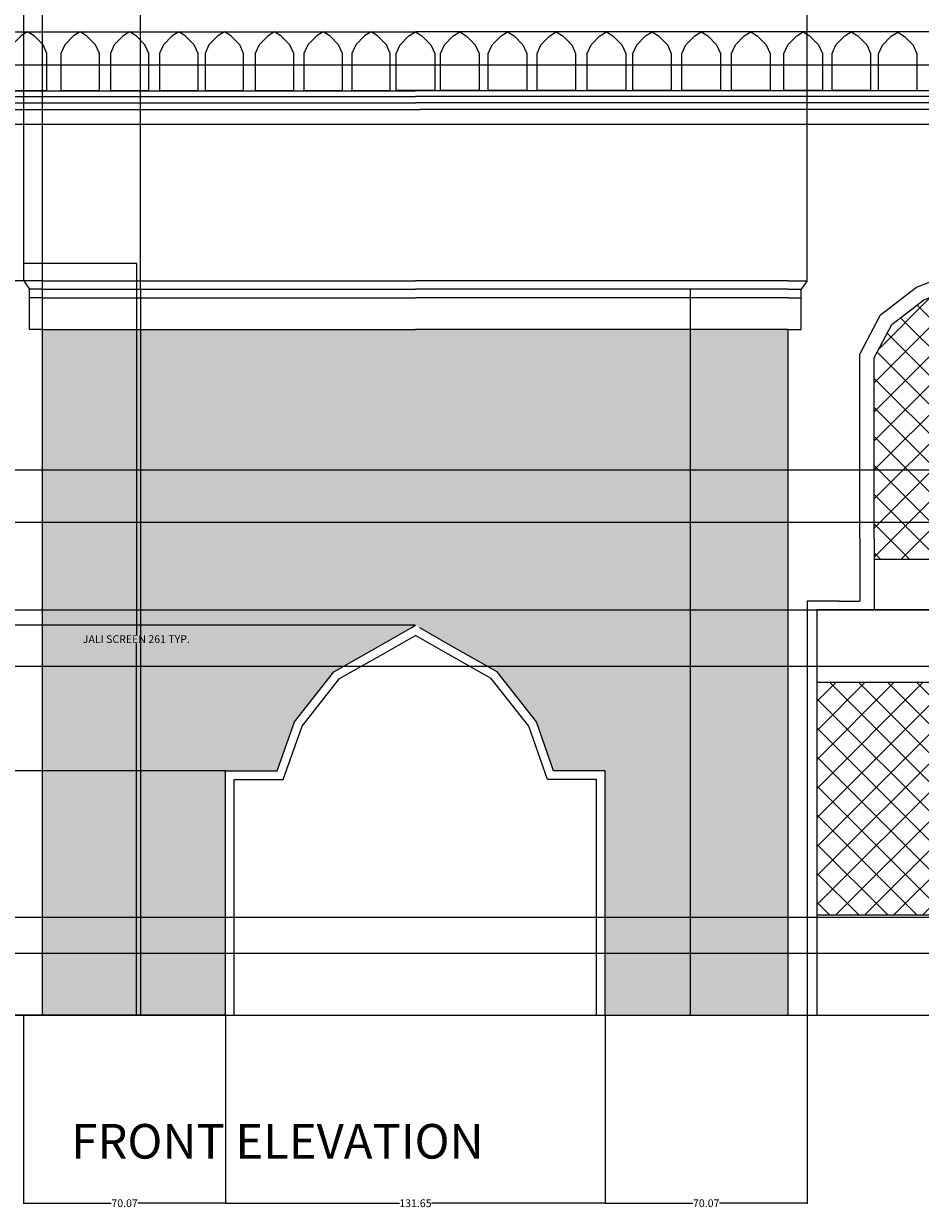
# Model space of a CAD drawing. Units: inches. Extents: x 2 to 1442, y 20 to 729.
# Tile 4 of 8: x 586 to 897, y 20 to 431. Entities that reach past the tile are written whole.
import ezdxf

# ---------------------------------------------------------------- set-up
doc = ezdxf.new("R2010")
doc.units = ezdxf.units.IN
doc.header["$MEASUREMENT"] = 0
for name, color, linetype, lineweight in [('A-ANNO-DIMS', 2, 'Continuous', 18), ('A-ANNO-TEXT', 7, 'Continuous', 25), ('A-ELEV', 7, 'Continuous', 25), ('A-GLAZ', 4, 'Continuous', 18), ('A-GLAZ-PATT', 9, 'Continuous', 13), ('A-WALL-PATT', 8, 'Continuous', 13)]:
    doc.layers.add(name, color=color, linetype=linetype, lineweight=lineweight)
doc.styles.get("Standard").update_dxf_attribs({"font": 'arial.ttf'})
doc.dimstyles.get("Standard").update_dxf_attribs({"dimtxt": 2.6875, "dimasz": 0.18, "dimexe": 0.18, "dimexo": 0.0625, "dimgap": 0.09, "dimtad": 0, "dimtih": 1, "dimtoh": 1, "dimdec": 4, "dimzin": 0, "dimdsep": 46, "dimlunit": 4, "dimtxsty": 'Standard', "dimcen": 0.09, "dimadec": 0, "dimazin": 0, "dimtfac": 1, "dimtdec": 4, "dimtofl": 0, "dimtmove": 0, "dimatfit": 3, "dimfxl": 1, "dimtolj": 1, "dimtzin": 0, "dimarcsym": 0})

# ---------------------------------------------------------------- blocks, each defined once
blk = doc.blocks.new('WIN-JALI-PANEL')
for p, q in [((17.71, 144.52), (17.71, 165.38)), ((22.71, 165.38), (22.71, 158.15)), ((95.66, 165.25), (95.66, 158.15)), ((100.66, 165.25), (100.66, 143.52)), ((95.66, 158.15), (22.71, 158.15)), ((22.71, 158.15), (22.71, 140.52)), ((95.66, 158.15), (95.66, 140.52)), ((0, 0), (0, 144.52)), ((7.01, 144.52), (0, 144.52)), ((7.01, 144.52), (17.71, 144.52)), ((107.81, 143.52), (100.66, 143.52)), ((107.81, 143.52), (118.87, 143.52)), ((118.87, 143.52), (118.87, 100.88)), ((118.87, 100.88), (118.87, 0))]:
    blk.add_line(p, q)
for points in [[(100.66, 165.25), (100.66, 224.45), (100.65, 229.2), (93.44, 242.86), (80.93, 252.42), (59.66, 260.79), (38.39, 252.42), (25.88, 242.86), (17.71, 227.39), (17.71, 165.38)], [(95.66, 165.25), (95.66, 224.45), (95.66, 227.96), (89.53, 239.55), (78.45, 248.02), (59.66, 255.41), (40.87, 248.02), (29.79, 239.55), (22.71, 226.15), (22.71, 165.38)]]:
    blk.add_lwpolyline(points)
blk = doc.blocks.new('*D9')
at = {"layer": 'A-ANNO-DIMS', "color": 0, "lineweight": -2, "transparency": 16777216}
for p, q in [((585.99, 348.06), (625.22, 348.06)), ((625.04, 347.88), (625.04, 219.14)), ((625.04, 87.45), (625.04, 216.18)), ((585.99, 87.27), (625.22, 87.27))]:
    blk.add_line(p, q, dxfattribs=at)
at = {"layer": 'A-ANNO-DIMS', "color": 0, "transparency": 16777216}
for points in [[(625.01, 347.88), (625.07, 347.88), (625.04, 348.06)], [(625.01, 87.45), (625.07, 87.45), (625.04, 87.27)]]:
    blk.add_solid(points, dxfattribs=at)
at = {"layer": 'Defpoints', "color": 0, "transparency": 16777216}
for p in [(585.93, 348.06), (625.04, 348.06), (585.93, 87.27)]:
    blk.add_point(p, dxfattribs=at)
at = {"layer": 'A-ANNO-DIMS', "color": 0, "transparency": 16777216, "insert": (625.04, 217.66), "char_height": 2.6875, "attachment_point": 5}
blk.add_mtext('\\A1;JALI SCREEN 261 TYP.', dxfattribs=at)
blk = doc.blocks.new('*D21')
at = {"layer": 'A-ANNO-DIMS', "color": 0, "lineweight": -2, "transparency": 16777216}
for p, q in [((585.93, 87.21), (585.93, 21.84)), ((656, 87.21), (656, 21.84)), ((586.11, 22.02), (616.35, 22.02)), ((655.82, 22.02), (625.58, 22.02))]:
    blk.add_line(p, q, dxfattribs=at)
at = {"layer": 'A-ANNO-DIMS', "color": 0, "transparency": 16777216}
for points in [[(586.11, 22.05), (586.11, 21.99), (585.93, 22.02)], [(655.82, 22.05), (655.82, 21.99), (656, 22.02)]]:
    blk.add_solid(points, dxfattribs=at)
at = {"layer": 'Defpoints', "color": 0, "transparency": 16777216}
for p in [(585.93, 87.27), (656, 87.27), (656, 22.02)]:
    blk.add_point(p, dxfattribs=at)
at = {"layer": 'A-ANNO-DIMS', "color": 0, "transparency": 16777216, "insert": (620.96, 22.02), "char_height": 2.688, "attachment_point": 5}
blk.add_mtext('\\A1;70.07', dxfattribs=at)
blk = doc.blocks.new('*D22')
at = {"layer": 'A-ANNO-DIMS', "color": 0, "lineweight": -2, "transparency": 16777216}
for p, q in [((656, 87.21), (656, 21.84)), ((787.65, 87.21), (787.65, 21.84)), ((656.18, 22.02), (716.27, 22.02)), ((787.47, 22.02), (727.38, 22.02))]:
    blk.add_line(p, q, dxfattribs=at)
at = {"layer": 'A-ANNO-DIMS', "color": 0, "transparency": 16777216}
for points in [[(656.18, 22.05), (656.18, 21.99), (656, 22.02)], [(787.47, 22.05), (787.47, 21.99), (787.65, 22.02)]]:
    blk.add_solid(points, dxfattribs=at)
at = {"layer": 'Defpoints', "color": 0, "transparency": 16777216}
for p in [(656, 87.27), (787.65, 87.27), (787.65, 22.02)]:
    blk.add_point(p, dxfattribs=at)
at = {"layer": 'A-ANNO-DIMS', "color": 0, "transparency": 16777216, "insert": (721.83, 22.02), "char_height": 2.688, "attachment_point": 5}
blk.add_mtext('\\A1;131.65', dxfattribs=at)
blk = doc.blocks.new('*D23')
at = {"layer": 'A-ANNO-DIMS', "color": 0, "lineweight": -2, "transparency": 16777216}
for p, q in [((787.65, 87.21), (787.65, 21.84)), ((857.73, 87.21), (857.73, 21.84)), ((787.83, 22.02), (818.08, 22.02)), ((857.55, 22.02), (827.3, 22.02))]:
    blk.add_line(p, q, dxfattribs=at)
at = {"layer": 'A-ANNO-DIMS', "color": 0, "transparency": 16777216}
for points in [[(787.83, 22.05), (787.83, 21.99), (787.65, 22.02)], [(857.55, 22.05), (857.55, 21.99), (857.73, 22.02)]]:
    blk.add_solid(points, dxfattribs=at)
at = {"layer": 'Defpoints', "color": 0, "transparency": 16777216}
for p in [(787.65, 87.27), (857.73, 87.27), (857.73, 22.02)]:
    blk.add_point(p, dxfattribs=at)
at = {"layer": 'A-ANNO-DIMS', "color": 0, "transparency": 16777216, "insert": (822.69, 22.02), "char_height": 2.688, "attachment_point": 5}
blk.add_mtext('\\A1;70.07', dxfattribs=at)
blk = doc.blocks.new('*D33')
at = {"layer": 'A-ANNO-DIMS', "color": 0, "lineweight": -2, "transparency": 16777216}
for p, q in [((722.06, 661.5), (1436.55, 661.5)), ((1436.37, 661.32), (1436.37, 375.85)), ((1436.37, 87.45), (1436.37, 372.92)), ((1371.19, 87.27), (1436.55, 87.27))]:
    blk.add_line(p, q, dxfattribs=at)
at = {"layer": 'A-ANNO-DIMS', "color": 0, "transparency": 16777216}
for points in [[(1436.34, 661.32), (1436.4, 661.32), (1436.37, 661.5)], [(1436.34, 87.45), (1436.4, 87.45), (1436.37, 87.27)]]:
    blk.add_solid(points, dxfattribs=at)
at = {"layer": 'Defpoints', "color": 0, "transparency": 16777216}
for p in [(722, 661.5), (1436.37, 661.5), (1371.12, 87.27)]:
    blk.add_point(p, dxfattribs=at)
at = {"layer": 'A-ANNO-DIMS', "color": 0, "transparency": 16777216, "insert": (1436.37, 374.39), "char_height": 2.688, "attachment_point": 5}
blk.add_mtext('\\A1;574.2', dxfattribs=at)
blk = doc.blocks.new('*D50')
at = {"layer": 'A-ANNO-DIMS', "color": 0, "lineweight": -2, "transparency": 16777216}
for p, q in [((433.03, 108.8), (1436.55, 108.8)), ((1436.37, 108.62), (1436.37, 99.5)), ((1436.37, 87.45), (1436.37, 96.57)), ((433.03, 87.27), (1436.55, 87.27))]:
    blk.add_line(p, q, dxfattribs=at)
at = {"layer": 'A-ANNO-DIMS', "color": 0, "transparency": 16777216}
for points in [[(1436.34, 108.62), (1436.4, 108.62), (1436.37, 108.8)], [(1436.34, 87.45), (1436.4, 87.45), (1436.37, 87.27)]]:
    blk.add_solid(points, dxfattribs=at)
at = {"layer": 'Defpoints', "color": 0, "transparency": 16777216}
for p in [(432.97, 108.8), (1436.37, 108.8), (432.97, 87.27)]:
    blk.add_point(p, dxfattribs=at)
at = {"layer": 'A-ANNO-DIMS', "color": 0, "transparency": 16777216, "insert": (1436.37, 98.04), "char_height": 2.688, "attachment_point": 5}
blk.add_mtext('\\A1;21.53', dxfattribs=at)
blk = doc.blocks.new('*D51')
at = {"layer": 'A-ANNO-DIMS', "color": 0, "lineweight": -2, "transparency": 16777216}
for p, q in [((426.83, 227.79), (1436.55, 227.79)), ((1436.37, 227.61), (1436.37, 169.76)), ((1436.37, 108.98), (1436.37, 166.83)), ((433.03, 108.8), (1436.55, 108.8))]:
    blk.add_line(p, q, dxfattribs=at)
at = {"layer": 'A-ANNO-DIMS', "color": 0, "transparency": 16777216}
for points in [[(1436.34, 227.61), (1436.4, 227.61), (1436.37, 227.79)], [(1436.34, 108.98), (1436.4, 108.98), (1436.37, 108.8)]]:
    blk.add_solid(points, dxfattribs=at)
at = {"layer": 'Defpoints', "color": 0, "transparency": 16777216}
for p in [(426.77, 227.79), (1436.37, 227.79), (432.97, 108.8)]:
    blk.add_point(p, dxfattribs=at)
at = {"layer": 'A-ANNO-DIMS', "color": 0, "transparency": 16777216, "insert": (1436.37, 168.3), "char_height": 2.688, "attachment_point": 5}
blk.add_mtext('\\A1;118.99', dxfattribs=at)
blk = doc.blocks.new('*D52')
at = {"layer": 'A-ANNO-DIMS', "color": 0, "lineweight": -2, "transparency": 16777216}
for p, q in [((433.03, 258.25), (1436.55, 258.25)), ((1436.37, 258.07), (1436.37, 244.49)), ((1436.37, 227.97), (1436.37, 241.56)), ((426.83, 227.79), (1436.55, 227.79))]:
    blk.add_line(p, q, dxfattribs=at)
at = {"layer": 'A-ANNO-DIMS', "color": 0, "transparency": 16777216}
for points in [[(1436.34, 258.07), (1436.4, 258.07), (1436.37, 258.25)], [(1436.34, 227.97), (1436.4, 227.97), (1436.37, 227.79)]]:
    blk.add_solid(points, dxfattribs=at)
at = {"layer": 'Defpoints', "color": 0, "transparency": 16777216}
for p in [(432.97, 258.25), (1436.37, 258.25), (426.77, 227.79)]:
    blk.add_point(p, dxfattribs=at)
at = {"layer": 'A-ANNO-DIMS', "color": 0, "transparency": 16777216, "insert": (1436.37, 243.02), "char_height": 2.688, "attachment_point": 5}
blk.add_mtext('\\A1;30.464', dxfattribs=at)
blk = doc.blocks.new('*D53')
at = {"layer": 'A-ANNO-DIMS', "color": 0, "lineweight": -2, "transparency": 16777216}
for p, q in [((433.03, 276.44), (1436.55, 276.44)), ((1436.37, 276.26), (1436.37, 268.81)), ((1436.37, 258.43), (1436.37, 265.89)), ((433.03, 258.25), (1436.55, 258.25))]:
    blk.add_line(p, q, dxfattribs=at)
at = {"layer": 'A-ANNO-DIMS', "color": 0, "transparency": 16777216}
for points in [[(1436.34, 276.26), (1436.4, 276.26), (1436.37, 276.44)], [(1436.34, 258.43), (1436.4, 258.43), (1436.37, 258.25)]]:
    blk.add_solid(points, dxfattribs=at)
at = {"layer": 'Defpoints', "color": 0, "transparency": 16777216}
for p in [(432.97, 276.44), (1436.37, 276.44), (432.97, 258.25)]:
    blk.add_point(p, dxfattribs=at)
at = {"layer": 'A-ANNO-DIMS', "color": 0, "transparency": 16777216, "insert": (1436.37, 267.35), "char_height": 2.688, "attachment_point": 5}
blk.add_mtext('\\A1;18.19', dxfattribs=at)
blk = doc.blocks.new('*D55')
at = {"layer": 'A-ANNO-DIMS', "color": 0, "lineweight": -2, "transparency": 16777216}
for p, q in [((391.01, 416.82), (1436.55, 416.82)), ((1436.37, 416.64), (1436.37, 407.98)), ((1436.37, 396.4), (1436.37, 405.06)), ((394.77, 396.22), (1436.55, 396.22))]:
    blk.add_line(p, q, dxfattribs=at)
at = {"layer": 'A-ANNO-DIMS', "color": 0, "transparency": 16777216}
for points in [[(1436.34, 416.64), (1436.4, 416.64), (1436.37, 416.82)], [(1436.34, 396.4), (1436.4, 396.4), (1436.37, 396.22)]]:
    blk.add_solid(points, dxfattribs=at)
at = {"layer": 'Defpoints', "color": 0, "transparency": 16777216}
for p in [(390.95, 416.82), (1436.37, 416.82), (394.7, 396.22)]:
    blk.add_point(p, dxfattribs=at)
at = {"layer": 'A-ANNO-DIMS', "color": 0, "transparency": 16777216, "insert": (1436.37, 406.52), "char_height": 2.688, "attachment_point": 5}
blk.add_mtext('\\A1;20.605', dxfattribs=at)
blk = doc.blocks.new('*D60')
at = {"layer": 'A-ANNO-DIMS', "color": 0, "lineweight": -2, "transparency": 16777216}
for p, q in [((414.48, 208.27), (1436.55, 208.27)), ((1436.37, 208.09), (1436.37, 166.24)), ((1436.37, 121.46), (1436.37, 163.32)), ((414.48, 121.28), (1436.55, 121.28))]:
    blk.add_line(p, q, dxfattribs=at)
at = {"layer": 'A-ANNO-DIMS', "color": 0, "transparency": 16777216}
for points in [[(1436.34, 208.09), (1436.4, 208.09), (1436.37, 208.27)], [(1436.34, 121.46), (1436.4, 121.46), (1436.37, 121.28)]]:
    blk.add_solid(points, dxfattribs=at)
at = {"layer": 'Defpoints', "color": 0, "transparency": 16777216}
for p in [(414.42, 208.27), (1436.37, 208.27), (414.42, 121.28)]:
    blk.add_point(p, dxfattribs=at)
at = {"layer": 'A-ANNO-DIMS', "color": 0, "transparency": 16777216, "insert": (1436.37, 164.78), "char_height": 2.688, "attachment_point": 5}
blk.add_mtext('\\A1;86.99', dxfattribs=at)
blk = doc.blocks.new('*D71')
at = {"layer": 'A-ANNO-DIMS', "color": 0, "lineweight": -2, "transparency": 16777216}
for p, q in [((586, 342.05), (586, 726.93)), ((586.18, 726.75), (716.12, 726.75)), ((857.47, 726.75), (727.53, 726.75)), ((857.65, 342.05), (857.65, 726.93))]:
    blk.add_line(p, q, dxfattribs=at)
at = {"layer": 'A-ANNO-DIMS', "color": 0, "transparency": 16777216}
for points in [[(586.18, 726.78), (586.18, 726.72), (586, 726.75)], [(857.47, 726.78), (857.47, 726.72), (857.65, 726.75)]]:
    blk.add_solid(points, dxfattribs=at)
at = {"layer": 'Defpoints', "color": 0, "transparency": 16777216}
for p in [(857.65, 726.75), (586, 341.99), (857.65, 341.99)]:
    blk.add_point(p, dxfattribs=at)
at = {"layer": 'A-ANNO-DIMS', "color": 0, "transparency": 16777216, "insert": (721.83, 726.75), "char_height": 2.688, "attachment_point": 5}
blk.add_mtext('\\A1;271.65', dxfattribs=at)
blk = doc.blocks.new('*D72')
at = {"layer": 'A-ANNO-DIMS', "color": 0, "lineweight": -2, "transparency": 16777216}
for p, q in [((585.94, 341.99), (7.1, 341.99)), ((7.28, 341.81), (7.28, 216.09)), ((7.28, 87.45), (7.28, 213.17)), ((592.44, 87.27), (7.1, 87.27))]:
    blk.add_line(p, q, dxfattribs=at)
at = {"layer": 'A-ANNO-DIMS', "color": 0, "transparency": 16777216}
for points in [[(7.25, 341.81), (7.31, 341.81), (7.28, 341.99)], [(7.25, 87.45), (7.31, 87.45), (7.28, 87.27)]]:
    blk.add_solid(points, dxfattribs=at)
at = {"layer": 'Defpoints', "color": 0, "transparency": 16777216}
for p in [(7.28, 341.99), (586, 341.99), (592.5, 87.27)]:
    blk.add_point(p, dxfattribs=at)
at = {"layer": 'A-ANNO-DIMS', "color": 0, "transparency": 16777216, "insert": (7.28, 214.63), "char_height": 2.688, "attachment_point": 5}
blk.add_mtext('\\A1;254.7', dxfattribs=at)
blk = doc.blocks.new('*D73')
at = {"layer": 'A-ANNO-DIMS', "color": 0, "lineweight": -2, "transparency": 16777216}
for p, q in [((592.5, 325.06), (592.5, 726.93)), ((592.68, 726.75), (607.49, 726.75)), ((626.32, 726.75), (611.51, 726.75)), ((626.5, 339.05), (626.5, 726.93))]:
    blk.add_line(p, q, dxfattribs=at)
at = {"layer": 'A-ANNO-DIMS', "color": 0, "transparency": 16777216}
for points in [[(592.68, 726.78), (592.68, 726.72), (592.5, 726.75)], [(626.32, 726.78), (626.32, 726.72), (626.5, 726.75)]]:
    blk.add_solid(points, dxfattribs=at)
at = {"layer": 'Defpoints', "color": 0, "transparency": 16777216}
for p in [(626.5, 726.75), (626.5, 338.99), (592.5, 325)]:
    blk.add_point(p, dxfattribs=at)
at = {"layer": 'A-ANNO-DIMS', "color": 0, "transparency": 16777216, "insert": (609.5, 726.75), "char_height": 2.688, "attachment_point": 5}
blk.add_mtext('\\A1;34', dxfattribs=at)
blk = doc.blocks.new('*D74')
at = {"layer": 'A-ANNO-DIMS', "color": 0, "lineweight": -2, "transparency": 16777216}
for p, q in [((655.94, 172), (7.1, 172)), ((7.28, 171.82), (7.28, 131.1)), ((7.28, 87.45), (7.28, 128.17)), ((655.94, 87.27), (7.1, 87.27))]:
    blk.add_line(p, q, dxfattribs=at)
at = {"layer": 'A-ANNO-DIMS', "color": 0, "transparency": 16777216}
for points in [[(7.25, 171.82), (7.31, 171.82), (7.28, 172)], [(7.25, 87.45), (7.31, 87.45), (7.28, 87.27)]]:
    blk.add_solid(points, dxfattribs=at)
at = {"layer": 'Defpoints', "color": 0, "transparency": 16777216}
for p in [(656, 172), (7.28, 87.27), (656, 87.27)]:
    blk.add_point(p, dxfattribs=at)
at = {"layer": 'A-ANNO-DIMS', "color": 0, "transparency": 16777216, "insert": (7.28, 129.64), "char_height": 2.688, "attachment_point": 5}
blk.add_mtext('\\A1;84.73', dxfattribs=at)
blk = doc.blocks.new('*D75')
at = {"layer": 'A-ANNO-DIMS', "color": 0, "lineweight": -2, "transparency": 16777216}
for p, q in [((721.76, 222.5), (7.1, 222.5)), ((7.28, 222.32), (7.28, 198.71)), ((7.28, 172.18), (7.28, 195.79)), ((655.94, 172), (7.1, 172))]:
    blk.add_line(p, q, dxfattribs=at)
at = {"layer": 'A-ANNO-DIMS', "color": 0, "transparency": 16777216}
for points in [[(7.25, 222.32), (7.31, 222.32), (7.28, 222.5)], [(7.25, 172.18), (7.31, 172.18), (7.28, 172)]]:
    blk.add_solid(points, dxfattribs=at)
at = {"layer": 'Defpoints', "color": 0, "transparency": 16777216}
for p in [(7.28, 222.5), (721.83, 222.5), (656, 172)]:
    blk.add_point(p, dxfattribs=at)
at = {"layer": 'A-ANNO-DIMS', "color": 0, "transparency": 16777216, "insert": (7.28, 197.25), "char_height": 2.688, "attachment_point": 5}
blk.add_mtext('\\A1;50.5', dxfattribs=at)

msp = doc.modelspace()

# ---------------------------------------------------------------- hatches: boundary and pattern name
at = {"layer": 'A-GLAZ-PATT'}
h = msp.add_hatch(dxfattribs=at)
h.set_pattern_fill('ANSI37', color=256, scale=57)
h.paths.add_polyline_path([(916.9314, 342.6839), (898.144, 335.2949), (887.0591, 326.8249), (880.9371, 315.2306), (880.9314, 311.7186), (880.9314, 252.5179), (880.9314, 245.4201), (953.8787, 245.4201), (953.8787, 252.6544), (953.8787, 313.4256), (946.8037, 326.8249), (935.7187, 335.2949)])
h.paths.add_polyline_path([(861.0256, 202.5842), (861.0256, 121.871), (972.8371, 121.871), (972.8371, 202.5842)])
at = {"layer": 'A-WALL-PATT'}
h = msp.add_hatch(dxfattribs=at)
h.set_pattern_fill('BRASS', color=256, scale=12)
h.paths.add_polyline_path([(721.8257, 325), (626.5, 325), (626.5, 87.2714), (656, 87.2714), (656, 172), (673.8743, 172), (679.8349, 188.9649), (693.5082, 206.3195), (709.021, 215.1101), (720.3466, 221.528), (721.8257, 222.5)])
h.paths.add_polyline_path([(626.5, 325), (592.5, 325), (592.5, 87.2714), (626.5, 87.2714)])
h = msp.add_hatch(dxfattribs=at)
h.set_pattern_fill('BRASS', color=256, scale=12)
h.paths.add_polyline_path([(721.8257, 325), (817.1514, 325), (817.1514, 87.2714), (787.6514, 87.2714), (787.6514, 172), (769.7771, 172), (763.8165, 188.9649), (750.1431, 206.3195), (734.6304, 215.1101), (723.3047, 221.528), (721.8257, 222.5)])
h.paths.add_polyline_path([(817.1514, 325), (851.1514, 325), (851.1514, 87.2714), (817.1514, 87.2714)])

# ---------------------------------------------------------------- linework, layer by layer
at = {"layer": 'A-ELEV'}
for p, q in [((432.9658, 428.3137), (716.9683, 428.3137)), ((716.9683, 428.3137), (721.8257, 428.3137)), ((726.6831, 428.3137), (721.8257, 428.3137)), ((1010.6856, 428.3137), (726.6831, 428.3137)), ((432.9658, 407.8873), (718.0964, 407.8873)), ((718.0964, 407.8873), (721.8257, 407.8873)), ((725.555, 407.8873), (721.8257, 407.8873)), ((1010.6856, 407.8873), (725.555, 407.8873)), ((432.9658, 405.9114), (715.3657, 405.9114)), ((432.9658, 403.6578), (721.8257, 403.6578)), ((715.3657, 405.9114), (721.8257, 405.9114)), ((728.2857, 405.9114), (721.8257, 405.9114)), ((1010.6856, 403.6578), (721.8257, 403.6578)), ((1010.6856, 405.9114), (728.2857, 405.9114)), ((432.9658, 401.3516), (720.2244, 401.3516)), ((720.2244, 401.3516), (721.8257, 401.3516)), ((721.8257, 401.3516), (723.427, 401.3516)), ((1010.6856, 401.3516), (723.427, 401.3516)), ((592.5, 341.9894), (586, 341.9894)), ((586, 341.9894), (588, 339)), ((592.5, 341.9894), (721.8257, 341.9894)), ((851.1514, 341.9894), (721.8257, 341.9894)), ((851.1514, 341.9894), (857.6514, 341.9894)), ((857.6514, 341.9894), (855.6514, 339)), ((588, 325), (588, 339)), ((592.5, 338.9894), (588, 339)), ((592.5, 338.9894), (721.8257, 338.9894)), ((626.5, 338.9894), (626.5, 87.2714)), ((851.1514, 338.9894), (721.8257, 338.9894)), ((817.1514, 338.9894), (817.1514, 87.2714)), ((851.1514, 338.9894), (855.6514, 339)), ((855.6514, 325), (855.6514, 339)), ((592.5, 335.9894), (588, 335.9894)), ((592.5, 335.9894), (721.8257, 335.9894)), ((851.1514, 335.9894), (721.8257, 335.9894)), ((851.1514, 335.9894), (855.6514, 335.9894)), ((592.5, 325), (588, 325)), ((592.5, 87.2714), (592.5, 325)), ((592.5, 325), (721.8257, 325)), ((851.1514, 325), (721.8257, 325)), ((851.1514, 87.2714), (851.1514, 325)), ((851.1514, 325), (855.6514, 325)), ((972.8371, 202.5842), (861.0256, 202.5842)), ((972.8371, 121.871), (861.0256, 121.871)), ((72.5272, 87.2714), (721.8257, 87.2714)), ((721.8257, 87.2714), (1371.1242, 87.2714))]:
    msp.add_line(p, q, dxfattribs=at)
for points in [[(594.0231, 420.8293), (592.6681, 423.7959), (589.5815, 426.88), (587.3386, 428.3137), (585.0958, 426.88), (582.0092, 423.7959), (580.6542, 420.8293), (580.6542, 407.9694), (594.0231, 407.9694)], [(612.2028, 420.8293), (610.8477, 423.7959), (607.7612, 426.88), (605.5183, 428.3137), (603.2754, 426.88), (600.1889, 423.7959), (598.8338, 420.8293), (598.8338, 407.9694), (612.2028, 407.9694)], [(629.3831, 420.8293), (628.0281, 423.7959), (624.9415, 426.88), (622.6986, 428.3137), (620.4558, 426.88), (617.3692, 423.7959), (616.0142, 420.8293), (616.0142, 407.9694), (629.3831, 407.9694)], [(646.4314, 420.8293), (645.0763, 423.7959), (641.9898, 426.88), (639.7469, 428.3137), (637.504, 426.88), (634.4175, 423.7959), (633.0624, 420.8293), (633.0624, 407.9694), (646.4314, 407.9694)], [(662.2457, 420.8293), (660.8906, 423.7959), (657.8041, 426.88), (655.5612, 428.3137), (653.3183, 426.88), (650.2318, 423.7959), (648.8767, 420.8293), (648.8767, 407.9694), (662.2457, 407.9694)], [(679.6382, 420.8293), (678.2832, 423.7959), (675.1966, 426.88), (672.9537, 428.3137), (670.7109, 426.88), (667.6243, 423.7959), (666.2693, 420.8293), (666.2693, 407.9694), (679.6382, 407.9694)], [(696.5456, 420.8293), (695.1905, 423.7959), (692.104, 426.88), (689.8611, 428.3137), (687.6182, 426.88), (684.5317, 423.7959), (683.1766, 420.8293), (683.1766, 407.9694), (696.5456, 407.9694)], [(713.1257, 420.8293), (711.7706, 423.7959), (708.6841, 426.88), (706.4412, 428.3137), (704.1983, 426.88), (701.1118, 423.7959), (699.7567, 420.8293), (699.7567, 407.9694), (713.1257, 407.9694)], [(715.1412, 420.8293), (716.4963, 423.7959), (719.5828, 426.88), (721.8257, 428.3137), (724.0686, 426.88), (727.1551, 423.7959), (728.5102, 420.8293), (728.5102, 407.9694), (715.1412, 407.9694)], [(730.5257, 420.8293), (731.8807, 423.7959), (734.9673, 426.88), (737.2102, 428.3137), (739.453, 426.88), (742.5396, 423.7959), (743.8946, 420.8293), (743.8946, 407.9694), (730.5257, 407.9694)], [(747.1058, 420.8293), (748.4609, 423.7959), (751.5474, 426.88), (753.7903, 428.3137), (756.0332, 426.88), (759.1197, 423.7959), (760.4748, 420.8293), (760.4748, 407.9694), (747.1058, 407.9694)], [(764.0132, 420.8293), (765.3682, 423.7959), (768.4548, 426.88), (770.6976, 428.3137), (772.9405, 426.88), (776.0271, 423.7959), (777.3821, 420.8293), (777.3821, 407.9694), (764.0132, 407.9694)], [(781.4057, 420.8293), (782.7608, 423.7959), (785.8473, 426.88), (788.0902, 428.3137), (790.3331, 426.88), (793.4196, 423.7959), (794.7747, 420.8293), (794.7747, 407.9694), (781.4057, 407.9694)], [(797.22, 420.8293), (798.575, 423.7959), (801.6616, 426.88), (803.9045, 428.3137), (806.1473, 426.88), (809.2339, 423.7959), (810.5889, 420.8293), (810.5889, 407.9694), (797.22, 407.9694)], [(814.2683, 420.8293), (815.6233, 423.7959), (818.7099, 426.88), (820.9527, 428.3137), (823.1956, 426.88), (826.2822, 423.7959), (827.6372, 420.8293), (827.6372, 407.9694), (814.2683, 407.9694)], [(831.4486, 420.8293), (832.8036, 423.7959), (835.8902, 426.88), (838.1331, 428.3137), (840.3759, 426.88), (843.4625, 423.7959), (844.8175, 420.8293), (844.8175, 407.9694), (831.4486, 407.9694)], [(849.6283, 420.8293), (850.9833, 423.7959), (854.0699, 426.88), (856.3127, 428.3137), (858.5556, 426.88), (861.6422, 423.7959), (862.9972, 420.8293), (862.9972, 407.9694), (849.6283, 407.9694)], [(866.3368, 420.8293), (867.6919, 423.7959), (870.7784, 426.88), (873.0213, 428.3137), (875.2642, 426.88), (878.3507, 423.7959), (879.7058, 420.8293), (879.7058, 407.9694), (866.3368, 407.9694)], [(882.4214, 420.7031), (883.7765, 423.6697), (886.863, 426.7538), (889.1059, 428.1874), (891.3488, 426.7538), (894.4353, 423.6697), (895.7904, 420.7031), (895.7904, 407.8432), (882.4214, 407.8432)], [(972.8371, 227.7901), (861.0256, 227.7901), (861.0256, 87.2714), (972.8371, 87.2714)]]:
    msp.add_lwpolyline(points, close=True, dxfattribs=at)
for points in [[(720.3466, 221.528), (721.8257, 222.5)], [(656, 87.2714), (656, 172), (673.8743, 172), (679.8349, 188.9649), (693.5082, 206.3195), (709.021, 215.1101), (720.3466, 221.528)], [(659, 87.2714), (659, 169), (676, 169), (682.5, 187.5), (695.5, 204), (710.5, 212.5), (721.8257, 218.9179)], [(784.6514, 87.2714), (784.6514, 169), (767.6514, 169), (761.1514, 187.5), (748.1514, 204), (733.1514, 212.5), (721.8257, 218.9179)], [(787.6514, 87.2714), (787.6514, 172), (769.7771, 172), (763.8165, 188.9649), (750.1431, 206.3195), (734.6304, 215.1101), (723.3047, 221.528)]]:
    msp.add_lwpolyline(points, dxfattribs=at)

# ---------------------------------------------------------------- block references
at = {"layer": 'A-GLAZ', "extrusion": (0, 0, -1), "zscale": -1}
msp.add_blockref('WIN-JALI-PANEL', (-976.5934, 87.271), dxfattribs=at)

# ---------------------------------------------------------------- texts
at = {"layer": 'A-ANNO-TEXT', "insert": (602.5, 49.5), "char_height": 12, "attachment_point": 1}
msp.add_mtext_dynamic_manual_height_columns('FRONT ELEVATION', width=273, gutter_width=1, heights=[0], dxfattribs=at)

# ---------------------------------------------------------------- dimensions: what is measured, and where the dimension line sits
at = {"layer": 'A-ANNO-DIMS'}
for base, p1, p2, override, picture, middle in [((857.6514, 726.75), (586, 341.9894), (857.6514, 341.9894), {"dimdec": 2, "dimlfac": 1, "dimrnd": 0, "dimzin": 0, "dimdsep": 46, "dimlunit": 2}, '*D71', (721.8257, 726.75)), ((626.5, 726.75), (592.5, 325), (626.5, 338.9894), {"dimdec": 0, "dimlfac": 1, "dimrnd": 0, "dimzin": 0, "dimdsep": 46, "dimlunit": 2}, '*D73', (609.5, 726.75)), ((656, 22.0214), (585.9257, 87.2714), (656, 87.2714), {"dimdec": 2, "dimlfac": 1, "dimrnd": 0, "dimzin": 0, "dimdsep": 46, "dimlunit": 2}, '*D21', (620.9629, 22.0214)), ((787.6514, 22.0214), (656, 87.2714), (787.6514, 87.2714), {"dimdec": 2, "dimlfac": 1, "dimrnd": 0, "dimzin": 0, "dimdsep": 46, "dimlunit": 2}, '*D22', (721.8257, 22.0214)), ((857.7256, 22.0214), (787.6514, 87.2714), (857.7256, 87.2714), {"dimdec": 2, "dimlfac": 1, "dimrnd": 0, "dimzin": 0, "dimdsep": 46, "dimlunit": 2}, '*D23', (822.6885, 22.0214))]:
    dim = msp.add_linear_dim(base=base, p1=p1, p2=p2, dimstyle='Standard', override=override, dxfattribs=at)
    dim.commit()
    dim.dimension.update_dxf_attribs({"geometry": picture, "text_midpoint": middle})
for base, p1, p2, override, picture, middle in [((1436.3742, 661.5), (1371.1242, 87.2714), (722, 661.5), {"dimdec": 1, "dimlfac": 1, "dimrnd": 0, "dimzin": 0, "dimdsep": 46, "dimlunit": 2}, '*D33', (1436.3742, 374.3857)), ((1436.3742, 416.8211), (394.7029, 396.2159), (390.9514, 416.8211), {"dimdec": 3, "dimlfac": 1, "dimrnd": 0, "dimzin": 0, "dimdsep": 46, "dimlunit": 2}, '*D55', (1436.3742, 406.5185)), ((7.2772, 341.9894), (592.5, 87.2714), (586, 341.9894), {"dimdec": 1, "dimlfac": 1, "dimrnd": 0, "dimzin": 0, "dimdsep": 46, "dimlunit": 2}, '*D72', (7.2772, 214.6304)), ((1436.3742, 276.443), (432.9658, 258.2539), (432.9658, 276.443), {"dimdec": 2, "dimlfac": 1, "dimrnd": 0, "dimzin": 0, "dimdsep": 46, "dimlunit": 2}, '*D53', (1436.3742, 267.3485)), ((1436.3742, 258.2539), (426.7688, 227.7901), (432.9658, 258.2539), {"dimdec": 3, "dimlfac": 1, "dimrnd": 0, "dimzin": 0, "dimdsep": 46, "dimlunit": 2}, '*D52', (1436.3742, 243.022)), ((1436.3742, 227.7901), (432.9658, 108.8033), (426.7688, 227.7901), {"dimdec": 2, "dimlfac": 1, "dimrnd": 0, "dimzin": 0, "dimdsep": 46, "dimlunit": 2}, '*D51', (1436.3742, 168.2967)), ((7.2772, 222.5), (656, 172), (721.8257, 222.5), {"dimdec": 1, "dimlfac": 1, "dimrnd": 0, "dimzin": 0, "dimdsep": 46, "dimlunit": 2}, '*D75', (7.2772, 197.25)), ((1436.3742, 208.2722), (414.4218, 121.2842), (414.4218, 208.2722), {"dimdec": 2, "dimlfac": 1, "dimrnd": 0, "dimzin": 0, "dimdsep": 46, "dimlunit": 2}, '*D60', (1436.3742, 164.7782)), ((7.2772, 87.2714), (656, 172), (656, 87.2714), {"dimdec": 2, "dimlfac": 1, "dimrnd": 0, "dimzin": 0, "dimdsep": 46, "dimlunit": 2}, '*D74', (7.2772, 129.6357)), ((1436.3742, 108.8033), (432.9658, 87.2714), (432.9658, 108.8033), {"dimdec": 2, "dimlfac": 1, "dimrnd": 0, "dimzin": 0, "dimdsep": 46, "dimlunit": 2}, '*D50', (1436.3742, 98.0373))]:
    dim = msp.add_linear_dim(base=base, p1=p1, p2=p2, angle=90, dimstyle='Standard', override=override, dxfattribs=at)
    dim.commit()
    dim.dimension.update_dxf_attribs({"geometry": picture, "text_midpoint": middle})
dim = msp.add_linear_dim(base=(625.0435, 348.0567), p1=(585.9257, 87.2714), p2=(585.9257, 348.0567), angle=90, text='JALI SCREEN <> TYP.', dimstyle='Standard', override={"dimdec": 0, "dimrnd": 0, "dimzin": 0, "dimlunit": 2}, dxfattribs=at)
dim.commit()
dim.dimension.update_dxf_attribs({"geometry": '*D9', "text_midpoint": (625.0435, 217.664)})

doc.saveas('drawing.dxf')
